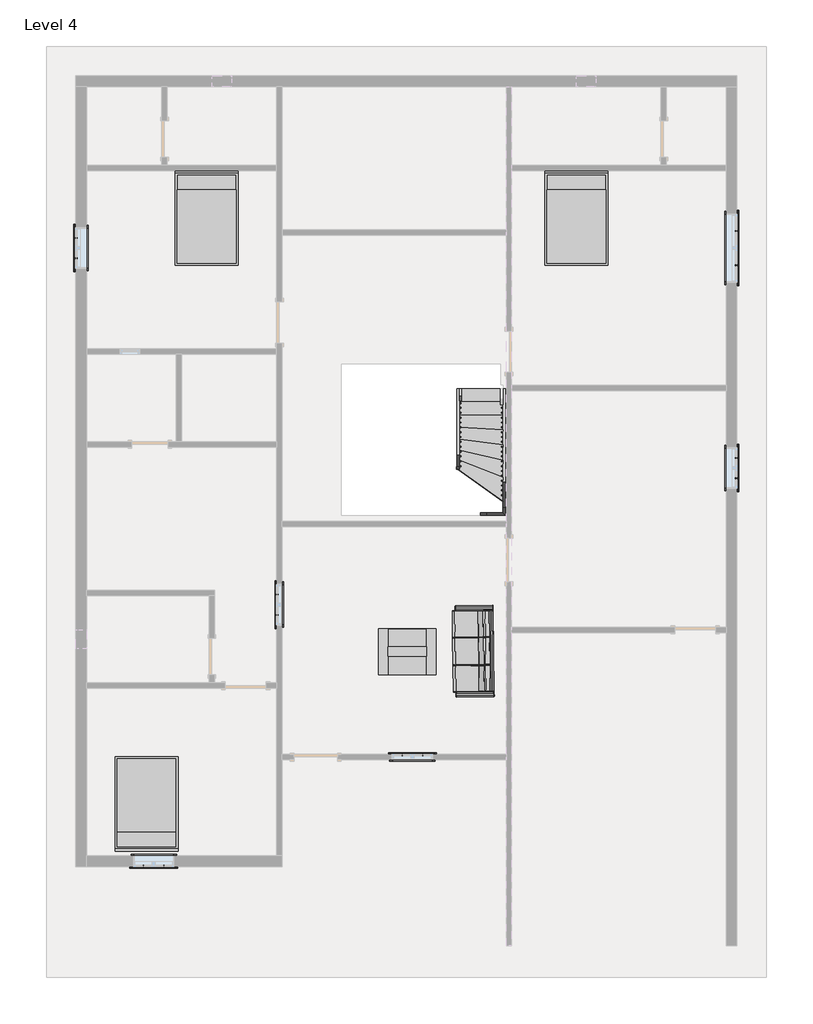
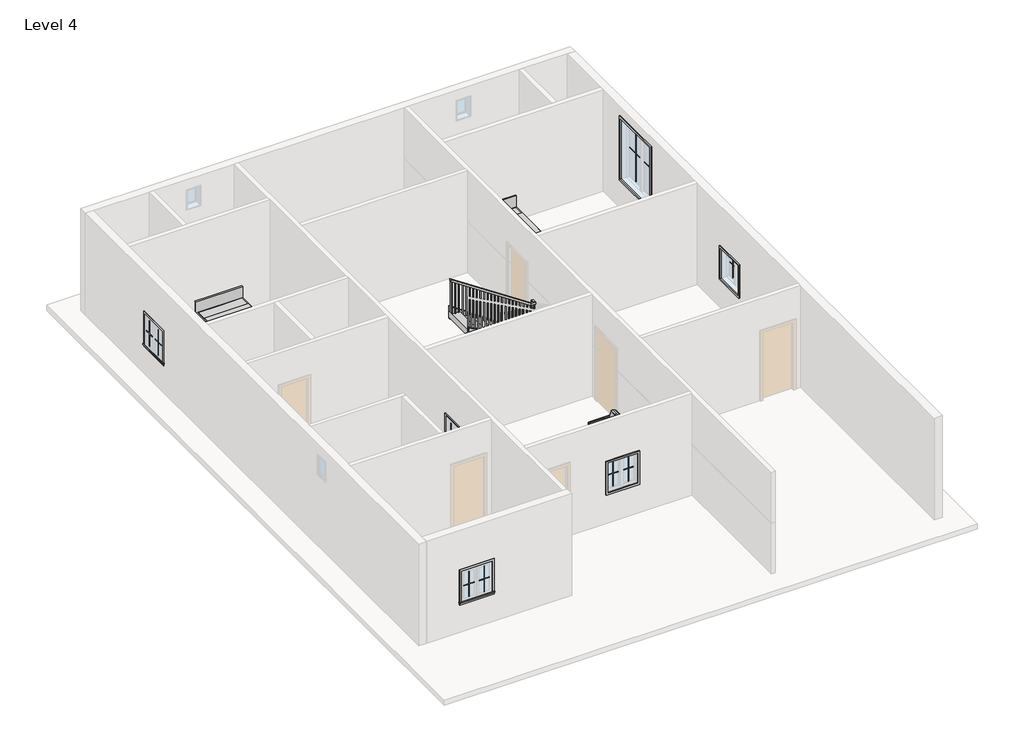
# One storey, part 3 of 3: 24 proxies, 6 members, 5 furniture elements, 1 railing, 1 stair flight.
"""IFC4 building model written with IfcOpenShell, lengths in millimetres."""

from ifc_helpers import new_model, si_unit, frame, origin, place, context, project, spatial, polyline, outline, extrude, faceted_brep, transform, mapped, element, save
from components import muntin_pattern_2x2_muntin_pattern_2x2_b3fe6957, muntin_pattern_2x2_muntin_pattern_2x2_3e0ecaf2, muntin_pattern_2x2_muntin_pattern_2x2_bff912c5, muntin_pattern_2x2_muntin_pattern_2x2_c2194282, trim_window_exterior_flat_with_sill_41619996, trim_window_exterior_flat_with_sill_e04b3088, trim_window_interior_flat_picture_frame_51c85655, trim_window_interior_flat_picture_frame_2a7685fe, furniture_2fc85b74, furniture_29a9adb8, furniture_57072a26, bed_17739_bed_17739_15c61121, wood_and_glass_coffee_table_17065_wood_and_glass_coffee_dbc724b2, stair_flight_9178a8c5

model = new_model("IFC4")

# Units and contexts
model_context = context("Model", 3, world=origin())
ifc_project = project(units=[si_unit("LENGTHUNIT", "METRE", prefix="MILLI")], contexts=[model_context])

# Site, building, storey
site = spatial("IfcSite", under=ifc_project)
building = spatial("IfcBuilding", under=site)
storey = spatial("IfcBuildingStorey", under=building, Name="Level 4", Elevation=6400.8)

# Proxies
placement = place(None, origin())
muntin_pattern_2x2_muntin_pattern_2x2_shape = muntin_pattern_2x2_muntin_pattern_2x2_b3fe6957(model_context)
element("IfcBuildingElementProxy", 1, Name="Muntin Pattern_2x2 : Muntin Pattern_2x2", ObjectType="Muntin Pattern_2x2 : Muntin Pattern_2x2", at=placement, inside=storey, context=model_context, shape_type="MappedRepresentation", body=[
    mapped(muntin_pattern_2x2_muntin_pattern_2x2_shape, transform((-7494.1165084, 6600.4397623, 7385.05), x_axis=(0.0, 1.0, 0.0), y_axis=(-1.0, 0.0, 0.0), z_axis=(0.0, 0.0, 1.0))),
])
element("IfcBuildingElementProxy", 2, Name="Muntin Pattern_2x2 : Muntin Pattern_2x2", ObjectType="Muntin Pattern_2x2 : Muntin Pattern_2x2", at=placement, inside=storey, context=model_context, shape_type="MappedRepresentation", body=[
    mapped(muntin_pattern_2x2_muntin_pattern_2x2_shape, transform((-5651.0290084, -6136.0727377, 7385.05), x_axis=(-1.0, 0.0, 0.0), y_axis=(0.0, -1.0, 0.0), z_axis=(0.0, 0.0, 1.0))),
])
element("IfcBuildingElementProxy", 3, Name="Muntin Pattern_2x2 : Muntin Pattern_2x2", ObjectType="Muntin Pattern_2x2 : Muntin Pattern_2x2", at=placement, inside=storey, context=model_context, shape_type="MappedRepresentation", body=[
    mapped(muntin_pattern_2x2_muntin_pattern_2x2_shape, transform((-656.7540084, -3805.6227377, 7385.05), x_axis=(1.0, 0.0, 0.0), y_axis=(0.0, 1.0, 0.0), z_axis=(0.0, 0.0, 1.0))),
])
element("IfcBuildingElementProxy", 4, Name="Muntin Pattern_2x2 : Muntin Pattern_2x2", ObjectType="Muntin Pattern_2x2 : Muntin Pattern_2x2", at=placement, inside=storey, context=model_context, shape_type="MappedRepresentation", body=[
    mapped(muntin_pattern_2x2_muntin_pattern_2x2_shape, transform((6355.2334916, 2418.9647623, 7385.05), x_axis=(0.0, -1.0, 0.0), y_axis=(1.0, 0.0, 0.0), z_axis=(0.0, 0.0, 1.0))),
])
element("IfcBuildingElementProxy", 5, Name="Muntin Pattern_2x2 : Muntin Pattern_2x2", ObjectType="Muntin Pattern_2x2 : Muntin Pattern_2x2", at=placement, inside=storey, context=model_context, shape_type="MappedRepresentation", body=[
    mapped(muntin_pattern_2x2_muntin_pattern_2x2_shape, transform((-3277.7165084, -873.5102377, 7385.05), x_axis=(0.0, 1.0, 0.0), y_axis=(-1.0, 0.0, 0.0), z_axis=(0.0, 0.0, 1.0))),
])
muntin_pattern_2x2_muntin_pattern_2x2_2_shape = muntin_pattern_2x2_muntin_pattern_2x2_3e0ecaf2(model_context)
element("IfcBuildingElementProxy", 6, Name="Muntin Pattern_2x2 : Muntin Pattern_2x2", ObjectType="Muntin Pattern_2x2 : Muntin Pattern_2x2", at=placement, inside=storey, context=model_context, shape_type="MappedRepresentation", body=[
    mapped(muntin_pattern_2x2_muntin_pattern_2x2_2_shape, transform((-7494.1165084, 7029.0647623, 7385.05), x_axis=(0.0, -1.0, 0.0), y_axis=(1.0, 0.0, 0.0), z_axis=(0.0, 0.0, 1.0))),
])
element("IfcBuildingElementProxy", 7, Name="Muntin Pattern_2x2 : Muntin Pattern_2x2", ObjectType="Muntin Pattern_2x2 : Muntin Pattern_2x2", at=placement, inside=storey, context=model_context, shape_type="MappedRepresentation", body=[
    mapped(muntin_pattern_2x2_muntin_pattern_2x2_2_shape, transform((-6079.6540084, -6136.0727377, 7385.05), x_axis=(1.0, 0.0, 0.0), y_axis=(0.0, 1.0, 0.0), z_axis=(0.0, 0.0, 1.0))),
])
element("IfcBuildingElementProxy", 8, Name="Muntin Pattern_2x2 : Muntin Pattern_2x2", ObjectType="Muntin Pattern_2x2 : Muntin Pattern_2x2", at=placement, inside=storey, context=model_context, shape_type="MappedRepresentation", body=[
    mapped(muntin_pattern_2x2_muntin_pattern_2x2_2_shape, transform((-228.1290084, -3805.6227377, 7385.05), x_axis=(-1.0, 0.0, 0.0), y_axis=(0.0, -1.0, 0.0), z_axis=(0.0, 0.0, 1.0))),
])
element("IfcBuildingElementProxy", 9, Name="Muntin Pattern_2x2 : Muntin Pattern_2x2", ObjectType="Muntin Pattern_2x2 : Muntin Pattern_2x2", at=placement, inside=storey, context=model_context, shape_type="MappedRepresentation", body=[
    mapped(muntin_pattern_2x2_muntin_pattern_2x2_2_shape, transform((6355.2334916, 1990.3397623, 7385.05), x_axis=(0.0, 1.0, 0.0), y_axis=(-1.0, 0.0, 0.0), z_axis=(0.0, 0.0, 1.0))),
])
element("IfcBuildingElementProxy", 10, Name="Muntin Pattern_2x2 : Muntin Pattern_2x2", ObjectType="Muntin Pattern_2x2 : Muntin Pattern_2x2", at=placement, inside=storey, context=model_context, shape_type="MappedRepresentation", body=[
    mapped(muntin_pattern_2x2_muntin_pattern_2x2_2_shape, transform((-3277.7165084, -444.8852377, 7385.05), x_axis=(0.0, -1.0, 0.0), y_axis=(1.0, 0.0, 0.0), z_axis=(0.0, 0.0, 1.0))),
])
muntin_pattern_2x2_muntin_pattern_2x2_3_shape = muntin_pattern_2x2_muntin_pattern_2x2_bff912c5(model_context)
element("IfcBuildingElementProxy", 11, Name="Muntin Pattern_2x2 : Muntin Pattern_2x2", ObjectType="Muntin Pattern_2x2 : Muntin Pattern_2x2", at=placement, inside=storey, context=model_context, shape_type="MappedRepresentation", body=[
    mapped(muntin_pattern_2x2_muntin_pattern_2x2_3_shape, transform((6355.2334916, 7175.1147623, 7385.05), x_axis=(0.0, -1.0, 0.0), y_axis=(1.0, 0.0, 0.0), z_axis=(0.0, 0.0, 1.0))),
])
muntin_pattern_2x2_muntin_pattern_2x2_4_shape = muntin_pattern_2x2_muntin_pattern_2x2_c2194282(model_context)
element("IfcBuildingElementProxy", 12, Name="Muntin Pattern_2x2 : Muntin Pattern_2x2", ObjectType="Muntin Pattern_2x2 : Muntin Pattern_2x2", at=placement, inside=storey, context=model_context, shape_type="MappedRepresentation", body=[
    mapped(muntin_pattern_2x2_muntin_pattern_2x2_4_shape, transform((6355.2334916, 6454.3897623, 7385.05), x_axis=(0.0, 1.0, 0.0), y_axis=(-1.0, 0.0, 0.0), z_axis=(0.0, 0.0, 1.0))),
])
trim_window_exterior_flat_with_sill_shape = trim_window_exterior_flat_with_sill_41619996(model_context)
element("IfcBuildingElementProxy", 13, Name="Trim-Window-Exterior-Flat : with Sill", ObjectType="Trim-Window-Exterior-Flat : with Sill", at=placement, inside=storey, context=model_context, shape_type="MappedRepresentation", body=[
    mapped(trim_window_exterior_flat_with_sill_shape, transform((-7503.6415084, 6814.7522623, 8229.6), x_axis=(0.0, -1.0, 0.0), y_axis=(0.0, 0.0, 1.0), z_axis=(-1.0, 0.0, 0.0))),
])
element("IfcBuildingElementProxy", 14, Name="Trim-Window-Exterior-Flat : with Sill", ObjectType="Trim-Window-Exterior-Flat : with Sill", at=placement, inside=storey, context=model_context, shape_type="MappedRepresentation", body=[
    mapped(trim_window_exterior_flat_with_sill_shape, transform((-5865.3415084, -6145.5977377, 8229.6), x_axis=(1.0, 0.0, 0.0), y_axis=(0.0, 0.0, 1.0), z_axis=(0.0, -1.0, 0.0))),
])
element("IfcBuildingElementProxy", 15, Name="Trim-Window-Exterior-Flat : with Sill", ObjectType="Trim-Window-Exterior-Flat : with Sill", at=placement, inside=storey, context=model_context, shape_type="MappedRepresentation", body=[
    mapped(trim_window_exterior_flat_with_sill_shape, transform((-442.4415084, -3796.0977377, 8229.6), x_axis=(-1.0, 0.0, 0.0), y_axis=(0.0, 0.0, 1.0), z_axis=(0.0, 1.0, 0.0))),
])
element("IfcBuildingElementProxy", 16, Name="Trim-Window-Exterior-Flat : with Sill", ObjectType="Trim-Window-Exterior-Flat : with Sill", at=placement, inside=storey, context=model_context, shape_type="MappedRepresentation", body=[
    mapped(trim_window_exterior_flat_with_sill_shape, transform((6364.7584916, 2204.6522623, 8229.6), x_axis=(0.0, 1.0, 0.0), y_axis=(0.0, 0.0, 1.0), z_axis=(1.0, 0.0, 0.0))),
])
element("IfcBuildingElementProxy", 17, Name="Trim-Window-Exterior-Flat : with Sill", ObjectType="Trim-Window-Exterior-Flat : with Sill", at=placement, inside=storey, context=model_context, shape_type="MappedRepresentation", body=[
    mapped(trim_window_exterior_flat_with_sill_shape, transform((-3287.2415084, -659.1977377, 8229.6), x_axis=(0.0, -1.0, 0.0), y_axis=(0.0, 0.0, 1.0), z_axis=(-1.0, 0.0, 0.0))),
])
trim_window_exterior_flat_with_sill_2_shape = trim_window_exterior_flat_with_sill_e04b3088(model_context)
element("IfcBuildingElementProxy", 18, Name="Trim-Window-Exterior-Flat : with Sill", ObjectType="Trim-Window-Exterior-Flat : with Sill", at=placement, inside=storey, context=model_context, shape_type="MappedRepresentation", body=[
    mapped(trim_window_exterior_flat_with_sill_2_shape, transform((6364.7584916, 6814.7522623, 9144.0), x_axis=(0.0, 1.0, 0.0), y_axis=(0.0, 0.0, 1.0), z_axis=(1.0, 0.0, 0.0))),
])
trim_window_interior_flat_picture_frame_shape = trim_window_interior_flat_picture_frame_51c85655(model_context)
element("IfcBuildingElementProxy", 19, Name="Trim-Window-Interior-Flat : Picture Frame", ObjectType="Trim-Window-Interior-Flat : Picture Frame", at=placement, inside=storey, context=model_context, shape_type="MappedRepresentation", body=[
    mapped(trim_window_interior_flat_picture_frame_shape, transform((-7275.0415084, 6814.7522623, 8229.6), x_axis=(0.0, 1.0, 0.0), y_axis=(0.0, 0.0, 1.0), z_axis=(1.0, 0.0, 0.0))),
])
element("IfcBuildingElementProxy", 20, Name="Trim-Window-Interior-Flat : Picture Frame", ObjectType="Trim-Window-Interior-Flat : Picture Frame", at=placement, inside=storey, context=model_context, shape_type="MappedRepresentation", body=[
    mapped(trim_window_interior_flat_picture_frame_shape, transform((-5865.3415084, -5916.9977377, 8229.6), x_axis=(-1.0, 0.0, 0.0), y_axis=(0.0, 0.0, 1.0), z_axis=(0.0, 1.0, 0.0))),
])
element("IfcBuildingElementProxy", 21, Name="Trim-Window-Interior-Flat : Picture Frame", ObjectType="Trim-Window-Interior-Flat : Picture Frame", at=placement, inside=storey, context=model_context, shape_type="MappedRepresentation", body=[
    mapped(trim_window_interior_flat_picture_frame_shape, transform((-442.4415084, -3910.3977377, 8229.6), x_axis=(1.0, 0.0, 0.0), y_axis=(0.0, 0.0, 1.0), z_axis=(0.0, -1.0, 0.0))),
])
element("IfcBuildingElementProxy", 22, Name="Trim-Window-Interior-Flat : Picture Frame", ObjectType="Trim-Window-Interior-Flat : Picture Frame", at=placement, inside=storey, context=model_context, shape_type="MappedRepresentation", body=[
    mapped(trim_window_interior_flat_picture_frame_shape, transform((6136.1584916, 2204.6522623, 8229.6), x_axis=(0.0, -1.0, 0.0), y_axis=(0.0, 0.0, 1.0), z_axis=(-1.0, 0.0, 0.0))),
])
element("IfcBuildingElementProxy", 23, Name="Trim-Window-Interior-Flat : Picture Frame", ObjectType="Trim-Window-Interior-Flat : Picture Frame", at=placement, inside=storey, context=model_context, shape_type="MappedRepresentation", body=[
    mapped(trim_window_interior_flat_picture_frame_shape, transform((-3172.9415084, -659.1977377, 8229.6), x_axis=(0.0, 1.0, 0.0), y_axis=(0.0, 0.0, 1.0), z_axis=(1.0, 0.0, 0.0))),
])
trim_window_interior_flat_picture_frame_2_shape = trim_window_interior_flat_picture_frame_2a7685fe(model_context)
element("IfcBuildingElementProxy", 24, Name="Trim-Window-Interior-Flat : Picture Frame", ObjectType="Trim-Window-Interior-Flat : Picture Frame", at=placement, inside=storey, context=model_context, shape_type="MappedRepresentation", body=[
    mapped(trim_window_interior_flat_picture_frame_2_shape, transform((6136.1584916, 6814.7522623, 9144.0), x_axis=(0.0, -1.0, 0.0), y_axis=(0.0, 0.0, 1.0), z_axis=(-1.0, 0.0, 0.0))),
])

# Furniture
furniture_shape = furniture_2fc85b74(model_context)
furniture_2_shape = furniture_29a9adb8(model_context)
furniture_3_shape = furniture_57072a26(model_context)
element("IfcFurniture", 25, at=placement, inside=storey, context=model_context, shape_type="MappedRepresentation", body=[
    mapped(furniture_shape, transform((460.7695276, -1640.1238257, 6400.8), x_axis=(0.014042050983927294, -0.9999014055416489, 0.0), y_axis=(0.9999014055416489, 0.014042050983927294, 0.0), z_axis=(0.0, 0.0, 1.0))),
    mapped(furniture_2_shape, transform((460.7695276, -1640.1238257, 6400.8), x_axis=(0.014042050983927294, -0.9999014055416489, 0.0), y_axis=(0.9999014055416489, 0.014042050983927294, 0.0), z_axis=(0.0, 0.0, 1.0))),
    mapped(furniture_3_shape, transform((460.7695276, -1640.1238257, 6400.8), x_axis=(0.014042050983927294, -0.9999014055416489, 0.0), y_axis=(0.9999014055416489, 0.014042050983927294, 0.0), z_axis=(0.0, 0.0, 1.0))),
])
bed_17739_bed_17739_shape = bed_17739_bed_17739_15c61121(model_context)
element("IfcFurniture", 26, ObjectType="Bed_17739 : Bed_17739", at=placement, inside=storey, context=model_context, shape_type="MappedRepresentation", body=[
    mapped(bed_17739_bed_17739_shape, transform((-4754.0915084, 7424.3522623, 6400.8), x_axis=(1.0, 0.0, 0.0), y_axis=(0.0, 1.0, 0.0), z_axis=(0.0, 0.0, 1.0))),
])
element("IfcFurniture", 27, ObjectType="Bed_17739 : Bed_17739", at=placement, inside=storey, context=model_context, shape_type="MappedRepresentation", body=[
    mapped(bed_17739_bed_17739_shape, transform((2998.5366507, 7424.3522623, 6400.8), x_axis=(1.0, 0.0, 0.0), y_axis=(0.0, 1.0, 0.0), z_axis=(0.0, 0.0, 1.0))),
])
element("IfcFurniture", 28, ObjectType="Bed_17739 : Bed_17739", at=placement, inside=storey, context=model_context, shape_type="MappedRepresentation", body=[
    mapped(bed_17739_bed_17739_shape, transform((-6017.7415084, -4812.0977377, 6400.8), x_axis=(-1.0, 0.0, 0.0), y_axis=(0.0, -1.0, 0.0), z_axis=(0.0, 0.0, 1.0))),
])
wood_and_glass_coffee_table_17065_wood_and_glass_coffee_shape = wood_and_glass_coffee_table_17065_wood_and_glass_coffee_dbc724b2(model_context)
element("IfcFurniture", 29, ObjectType="Wood_and_Glass_Coffee_Table_17065 : Wood_and_Glass_Coffee_Table_17065", at=placement, inside=storey, context=model_context, shape_type="MappedRepresentation", body=[
    mapped(wood_and_glass_coffee_table_17065_wood_and_glass_coffee_shape, transform((-550.3915084, -1643.4477377, 6400.8), x_axis=(1.0, 0.0, 0.0), y_axis=(0.0, 1.0, 0.0), z_axis=(0.0, 0.0, 1.0))),
])

# Members
element("IfcMember", 30, ObjectType="Stringer - 2\" Width", at=placement, inside=storey, context=model_context, shape_type="SweptSolid", body=[
    extrude(outline(polyline([(3870.4222402, 6634.4789033), (3870.4222402, 6400.8), (3655.4968958, 6400.8), (1369.1992084, 7533.4067011), (1369.1992084, 7873.5572536), (3870.4222402, 6634.4789033)])), frame((1456.2084916, 0.0, 0.0), z_axis=(1.0, 0.0, 0.0), x_axis=(0.0, 1.0, 0.0)), (0.0, 0.0, 1.0), 50.8),
])
element("IfcMember", 31, ObjectType="Stringer - 2\" Width", at=placement, inside=storey, context=model_context, shape_type="SweptSolid", body=[
    extrude(outline(polyline([(1456.2084916, 1369.1992084), (1507.0084916, 1369.1992084), (1507.0084916, 1218.1652728), (1456.2084916, 1268.9652728), (1456.2084916, 1369.1992084)])), frame((0.0, 0.0, 7533.4067011), z_axis=(0.0, 0.0, 1.0), x_axis=(1.0, 0.0, 0.0)), (0.0, 0.0, 1.0), 340.1505525),
])
element("IfcMember", 32, ObjectType="Stringer - 2\" Width", at=placement, inside=storey, context=model_context, shape_type="SweptSolid", body=[
    extrude(outline(polyline([(1456.2084916, 1268.9652728), (1507.0084916, 1218.1652728), (1113.208453, 1218.1652728), (1113.208453, 1268.9652728), (1456.2084916, 1268.9652728)])), frame((0.0, 0.0, 7533.4067011), z_axis=(0.0, 0.0, 1.0), x_axis=(1.0, 0.0, 0.0)), (0.0, 0.0, 1.0), 340.1505525),
])
element("IfcMember", 33, ObjectType="Stringer - 2\" Width", at=placement, inside=storey, context=model_context, shape_type="SweptSolid", body=[
    extrude(outline(polyline([(3870.4222402, 6591.0545013), (3870.4222402, 6400.8), (3614.0281198, 6400.8), (2234.1652728, 7407.2313584), (2234.1652728, 7784.4921868), (3870.4222402, 6591.0545013)])), frame((491.0084916, 0.0, 0.0), z_axis=(1.0, 0.0, 0.0), x_axis=(0.0, 1.0, 0.0)), (0.0, 0.0, 1.0), 50.8),
])
element("IfcMember", 34, ObjectType="Stringer - 2\" Width", at=placement, inside=storey, context=model_context, shape_type="SweptSolid", body=[
    extrude(outline(polyline([(7558.9835681, 541.8084916), (7926.7965617, 541.8084916), (9517.7897736, -1813.7050583), (9149.97678, -1813.7050583), (7558.9835681, 541.8084916)])), frame((0.0, 2183.3652728, 0.0), z_axis=(0.0, 1.0, 0.0), x_axis=(0.0, 0.0, 1.0)), (0.0, 0.0, 1.0), 50.8),
])
element("IfcMember", 35, ObjectType="Stringer - 2\" Width", at=placement, inside=storey, context=model_context, shape_type="SweptSolid", body=[
    extrude(outline(polyline([(7533.4067011, 1113.208453), (7873.5572536, 1113.208453), (9464.7877281, -1813.7050583), (9124.6371756, -1813.7050583), (7533.4067011, 1113.208453)])), frame((0.0, 1218.1652728, 0.0), z_axis=(0.0, 1.0, 0.0), x_axis=(0.0, 0.0, 1.0)), (0.0, 0.0, 1.0), 50.8),
])

# Railing
element("IfcRailing", 36, ObjectType="Handrail - Rectangular", at=placement, inside=storey, context=model_context, shape_type="SolidModel", body=[
    faceted_brep([(592.6084916, 3870.4222402, 7484.5333333), (592.6084916, 3870.4222402, 7422.2674881), (541.8084916, 3870.4222402, 7422.2674881), (541.8084916, 3870.4222402, 7484.5333333), (592.6084916, 2259.5652728, 8626.2596781), (592.6084916, 2208.7652728, 8599.9993253), (541.8084916, 2208.7652728, 8599.9993253), (541.8084916, 2259.5652728, 8626.2596781), (592.6084916, 2259.5652728, 8843.0092282), (592.6084916, 2208.7652728, 8792.2092282), (541.8084916, 2208.7652728, 8792.2092282), (541.8084916, 2259.5652728, 8843.0092282), (592.6084916, 2132.5652728, 8843.0092282), (592.6084916, 2132.5652728, 8792.2092282), (541.8084916, 2183.3652728, 8792.2092282), (541.8084916, 2183.3652728, 8843.0092282), (465.6084916, 2132.5652728, 8843.0092282), (450.2220288, 2132.5652728, 8792.2092282), (450.2220288, 2183.3652728, 8792.2092282), (465.6084916, 2183.3652728, 8843.0092282), (-1813.7050583, 2132.5652728, 10363.2), (-1813.7050583, 2183.3652728, 10363.2), (-1813.7050583, 2183.3652728, 10302.1379811), (-1813.7050583, 2132.5652728, 10302.1379811)], [[[0, 1, 2, 3]], [[1, 0, 4, 5]], [[2, 1, 5, 6]], [[3, 2, 6, 7]], [[0, 3, 7, 4]], [[5, 4, 8, 9]], [[6, 5, 9, 10]], [[7, 6, 10, 11]], [[4, 7, 11, 8]], [[9, 8, 12, 13]], [[10, 9, 13, 14]], [[11, 10, 14, 15]], [[8, 11, 15, 12]], [[13, 12, 16, 17]], [[14, 13, 17, 18]], [[15, 14, 18, 19]], [[12, 15, 19, 16]], [[20, 21, 22, 23]], [[17, 16, 20, 23]], [[18, 17, 23, 22]], [[19, 18, 22, 21]], [[16, 19, 21, 20]]]),
    extrude(outline(polyline([(10266.3636891, -1760.0665084), (10279.0691083, -1779.1165084), (9279.4666667, -1779.1165084), (9279.4666667, -1760.0665084), (10266.3636891, -1760.0665084)])), frame((0.0, 2148.4402728, 0.0), z_axis=(0.0, 1.0, 0.0), x_axis=(0.0, 0.0, 1.0)), (0.0, 0.0, 1.0), 19.05),
    extrude(outline(polyline([(10198.6014532, -1658.4665084), (10211.3068724, -1677.5165084), (9279.4666667, -1677.5165084), (9279.4666667, -1658.4665084), (10198.6014532, -1658.4665084)])), frame((0.0, 2148.4402728, 0.0), z_axis=(0.0, 1.0, 0.0), x_axis=(0.0, 0.0, 1.0)), (0.0, 0.0, 1.0), 19.05),
    extrude(outline(polyline([(10130.8392173, -1556.8665084), (10143.5446365, -1575.9165084), (9279.4666667, -1575.9165084), (9279.4666667, -1556.8665084), (10130.8392173, -1556.8665084)])), frame((0.0, 2148.4402728, 0.0), z_axis=(0.0, 1.0, 0.0), x_axis=(0.0, 0.0, 1.0)), (0.0, 0.0, 1.0), 19.05),
    extrude(outline(polyline([(10062.9324687, -1455.2665084), (10075.6378879, -1474.3165084), (9110.1333333, -1474.3165084), (9110.1333333, -1455.2665084), (10062.9324687, -1455.2665084)])), frame((0.0, 2148.4402728, 0.0), z_axis=(0.0, 1.0, 0.0), x_axis=(0.0, 0.0, 1.0)), (0.0, 0.0, 1.0), 19.05),
    extrude(outline(polyline([(9995.1702328, -1353.6665084), (10007.875652, -1372.7165084), (9110.1333333, -1372.7165084), (9110.1333333, -1353.6665084), (9995.1702328, -1353.6665084)])), frame((0.0, 2148.4402728, 0.0), z_axis=(0.0, 1.0, 0.0), x_axis=(0.0, 0.0, 1.0)), (0.0, 0.0, 1.0), 19.05),
    extrude(outline(polyline([(9927.4079969, -1252.0665084), (9940.1134161, -1271.1165084), (9110.1333333, -1271.1165084), (9110.1333333, -1252.0665084), (9927.4079969, -1252.0665084)])), frame((0.0, 2148.4402728, 0.0), z_axis=(0.0, 1.0, 0.0), x_axis=(0.0, 0.0, 1.0)), (0.0, 0.0, 1.0), 19.05),
    extrude(outline(polyline([(9859.645761, -1150.4665084), (9872.3511802, -1169.5165084), (8940.8, -1169.5165084), (8940.8, -1150.4665084), (9859.645761, -1150.4665084)])), frame((0.0, 2148.4402728, 0.0), z_axis=(0.0, 1.0, 0.0), x_axis=(0.0, 0.0, 1.0)), (0.0, 0.0, 1.0), 19.05),
    extrude(outline(polyline([(9791.8835251, -1048.8665084), (9804.5889444, -1067.9165084), (8940.8, -1067.9165084), (8940.8, -1048.8665084), (9791.8835251, -1048.8665084)])), frame((0.0, 2148.4402728, 0.0), z_axis=(0.0, 1.0, 0.0), x_axis=(0.0, 0.0, 1.0)), (0.0, 0.0, 1.0), 19.05),
    extrude(outline(polyline([(9724.265802, -947.2665084), (9736.9712212, -966.3165084), (8771.4666667, -966.3165084), (8771.4666667, -947.2665084), (9724.265802, -947.2665084)])), frame((0.0, 2148.4402728, 0.0), z_axis=(0.0, 1.0, 0.0), x_axis=(0.0, 0.0, 1.0)), (0.0, 0.0, 1.0), 19.05),
    extrude(outline(polyline([(9656.5035661, -845.6665084), (9669.2089853, -864.7165084), (8771.4666667, -864.7165084), (8771.4666667, -845.6665084), (9656.5035661, -845.6665084)])), frame((0.0, 2148.4402728, 0.0), z_axis=(0.0, 1.0, 0.0), x_axis=(0.0, 0.0, 1.0)), (0.0, 0.0, 1.0), 19.05),
    extrude(outline(polyline([(9588.7413302, -744.0665084), (9601.4467495, -763.1165084), (8771.4666667, -763.1165084), (8771.4666667, -744.0665084), (9588.7413302, -744.0665084)])), frame((0.0, 2148.4402728, 0.0), z_axis=(0.0, 1.0, 0.0), x_axis=(0.0, 0.0, 1.0)), (0.0, 0.0, 1.0), 19.05),
    extrude(outline(polyline([(9520.9790943, -642.4665084), (9533.6845136, -661.5165084), (8602.1333333, -661.5165084), (8602.1333333, -642.4665084), (9520.9790943, -642.4665084)])), frame((0.0, 2148.4402728, 0.0), z_axis=(0.0, 1.0, 0.0), x_axis=(0.0, 0.0, 1.0)), (0.0, 0.0, 1.0), 19.05),
    extrude(outline(polyline([(9453.2168585, -540.8665084), (9465.9222777, -559.9165084), (8602.1333333, -559.9165084), (8602.1333333, -540.8665084), (9453.2168585, -540.8665084)])), frame((0.0, 2148.4402728, 0.0), z_axis=(0.0, 1.0, 0.0), x_axis=(0.0, 0.0, 1.0)), (0.0, 0.0, 1.0), 19.05),
    extrude(outline(polyline([(9385.3101098, -439.2665084), (9398.0155291, -458.3165084), (8602.1333333, -458.3165084), (8602.1333333, -439.2665084), (9385.3101098, -439.2665084)])), frame((0.0, 2148.4402728, 0.0), z_axis=(0.0, 1.0, 0.0), x_axis=(0.0, 0.0, 1.0)), (0.0, 0.0, 1.0), 19.05),
    extrude(outline(polyline([(9317.5478739, -337.6665084), (9330.2532932, -356.7165084), (8432.8, -356.7165084), (8432.8, -337.6665084), (9317.5478739, -337.6665084)])), frame((0.0, 2148.4402728, 0.0), z_axis=(0.0, 1.0, 0.0), x_axis=(0.0, 0.0, 1.0)), (0.0, 0.0, 1.0), 19.05),
    extrude(outline(polyline([(9249.7856381, -236.0665084), (9262.4910573, -255.1165084), (8432.8, -255.1165084), (8432.8, -236.0665084), (9249.7856381, -236.0665084)])), frame((0.0, 2148.4402728, 0.0), z_axis=(0.0, 1.0, 0.0), x_axis=(0.0, 0.0, 1.0)), (0.0, 0.0, 1.0), 19.05),
    extrude(outline(polyline([(9182.0234022, -134.4665084), (9194.7288214, -153.5165084), (8263.4666667, -153.5165084), (8263.4666667, -134.4665084), (9182.0234022, -134.4665084)])), frame((0.0, 2148.4402728, 0.0), z_axis=(0.0, 1.0, 0.0), x_axis=(0.0, 0.0, 1.0)), (0.0, 0.0, 1.0), 19.05),
    extrude(outline(polyline([(9114.2611663, -32.8665084), (9126.9665855, -51.9165084), (8263.4666667, -51.9165084), (8263.4666667, -32.8665084), (9114.2611663, -32.8665084)])), frame((0.0, 2148.4402728, 0.0), z_axis=(0.0, 1.0, 0.0), x_axis=(0.0, 0.0, 1.0)), (0.0, 0.0, 1.0), 19.05),
    extrude(outline(polyline([(9046.6434432, 68.7334916), (9059.3488624, 49.6834916), (8263.4666667, 49.6834916), (8263.4666667, 68.7334916), (9046.6434432, 68.7334916)])), frame((0.0, 2148.4402728, 0.0), z_axis=(0.0, 1.0, 0.0), x_axis=(0.0, 0.0, 1.0)), (0.0, 0.0, 1.0), 19.05),
    extrude(outline(polyline([(8978.8812073, 170.3334916), (8991.5866265, 151.2834916), (8094.1333333, 151.2834916), (8094.1333333, 170.3334916), (8978.8812073, 170.3334916)])), frame((0.0, 2148.4402728, 0.0), z_axis=(0.0, 1.0, 0.0), x_axis=(0.0, 0.0, 1.0)), (0.0, 0.0, 1.0), 19.05),
    extrude(outline(polyline([(8911.1189714, 271.9334916), (8923.8243906, 252.8834916), (8094.1333333, 252.8834916), (8094.1333333, 271.9334916), (8911.1189714, 271.9334916)])), frame((0.0, 2148.4402728, 0.0), z_axis=(0.0, 1.0, 0.0), x_axis=(0.0, 0.0, 1.0)), (0.0, 0.0, 1.0), 19.05),
    extrude(outline(polyline([(8843.3567355, 373.5334916), (8856.0621547, 354.4834916), (7924.8, 354.4834916), (7924.8, 373.5334916), (8843.3567355, 373.5334916)])), frame((0.0, 2148.4402728, 0.0), z_axis=(0.0, 1.0, 0.0), x_axis=(0.0, 0.0, 1.0)), (0.0, 0.0, 1.0), 19.05),
    extrude(outline(polyline([(8775.5944996, 475.1334916), (8788.2999189, 456.0834916), (7924.8, 456.0834916), (7924.8, 475.1334916), (8775.5944996, 475.1334916)])), frame((0.0, 2148.4402728, 0.0), z_axis=(0.0, 1.0, 0.0), x_axis=(0.0, 0.0, 1.0)), (0.0, 0.0, 1.0), 19.05),
    extrude(outline(polyline([(557.6834916, 2254.3472402), (576.7334916, 2254.3472402), (576.7334916, 2235.2972402), (557.6834916, 2235.2972402), (557.6834916, 2254.3472402)])), frame((0.0, 0.0, 7586.1333333), z_axis=(0.0, 0.0, 1.0), x_axis=(1.0, 0.0, 0.0)), (0.0, 0.0, 1.0), 1206.0758948),
    extrude(outline(polyline([(2336.8972402, 8509.1832902), (2355.9472402, 8495.6812306), (2355.9472402, 7586.1333333), (2336.8972402, 7586.1333333), (2336.8972402, 8509.1832902)])), frame((557.6834916, 0.0, 0.0), z_axis=(1.0, 0.0, 0.0), x_axis=(0.0, 1.0, 0.0)), (0.0, 0.0, 1.0), 19.05),
    extrude(outline(polyline([(2438.4972402, 8437.1723054), (2457.5472402, 8423.6702458), (2457.5472402, 7416.8), (2438.4972402, 7416.8), (2438.4972402, 8437.1723054)])), frame((557.6834916, 0.0, 0.0), z_axis=(1.0, 0.0, 0.0), x_axis=(0.0, 1.0, 0.0)), (0.0, 0.0, 1.0), 19.05),
    extrude(outline(polyline([(2540.0972402, 8365.1613206), (2559.1472402, 8351.6592609), (2559.1472402, 7416.8), (2540.0972402, 7416.8), (2540.0972402, 8365.1613206)])), frame((557.6834916, 0.0, 0.0), z_axis=(1.0, 0.0, 0.0), x_axis=(0.0, 1.0, 0.0)), (0.0, 0.0, 1.0), 19.05),
    extrude(outline(polyline([(2641.6972402, 8293.1503358), (2660.7472402, 8279.6482761), (2660.7472402, 7247.4666667), (2641.6972402, 7247.4666667), (2641.6972402, 8293.1503358)])), frame((557.6834916, 0.0, 0.0), z_axis=(1.0, 0.0, 0.0), x_axis=(0.0, 1.0, 0.0)), (0.0, 0.0, 1.0), 19.05),
    extrude(outline(polyline([(2743.2972402, 8221.139351), (2762.3472402, 8207.6372913), (2762.3472402, 7247.4666667), (2743.2972402, 7247.4666667), (2743.2972402, 8221.139351)])), frame((557.6834916, 0.0, 0.0), z_axis=(1.0, 0.0, 0.0), x_axis=(0.0, 1.0, 0.0)), (0.0, 0.0, 1.0), 19.05),
    extrude(outline(polyline([(2844.8972402, 8149.1283661), (2863.9472402, 8135.6263065), (2863.9472402, 7078.1333333), (2844.8972402, 7078.1333333), (2844.8972402, 8149.1283661)])), frame((557.6834916, 0.0, 0.0), z_axis=(1.0, 0.0, 0.0), x_axis=(0.0, 1.0, 0.0)), (0.0, 0.0, 1.0), 19.05),
    extrude(outline(polyline([(2946.4972402, 8077.1173813), (2965.5472402, 8063.6153217), (2965.5472402, 7078.1333333), (2946.4972402, 7078.1333333), (2946.4972402, 8077.1173813)])), frame((557.6834916, 0.0, 0.0), z_axis=(1.0, 0.0, 0.0), x_axis=(0.0, 1.0, 0.0)), (0.0, 0.0, 1.0), 19.05),
    extrude(outline(polyline([(3048.0972402, 8005.1063965), (3067.1472402, 7991.6043368), (3067.1472402, 6908.8), (3048.0972402, 6908.8), (3048.0972402, 8005.1063965)])), frame((557.6834916, 0.0, 0.0), z_axis=(1.0, 0.0, 0.0), x_axis=(0.0, 1.0, 0.0)), (0.0, 0.0, 1.0), 19.05),
    extrude(outline(polyline([(3149.6972402, 7933.0954117), (3168.7472402, 7919.593352), (3168.7472402, 6908.8), (3149.6972402, 6908.8), (3149.6972402, 7933.0954117)])), frame((557.6834916, 0.0, 0.0), z_axis=(1.0, 0.0, 0.0), x_axis=(0.0, 1.0, 0.0)), (0.0, 0.0, 1.0), 19.05),
    extrude(outline(polyline([(3251.2972402, 7861.0844268), (3270.3472402, 7847.5823672), (3270.3472402, 6908.8), (3251.2972402, 6908.8), (3251.2972402, 7861.0844268)])), frame((557.6834916, 0.0, 0.0), z_axis=(1.0, 0.0, 0.0), x_axis=(0.0, 1.0, 0.0)), (0.0, 0.0, 1.0), 19.05),
    extrude(outline(polyline([(3352.8972402, 7789.073442), (3371.9472402, 7775.5713824), (3371.9472402, 6739.4666667), (3352.8972402, 6739.4666667), (3352.8972402, 7789.073442)])), frame((557.6834916, 0.0, 0.0), z_axis=(1.0, 0.0, 0.0), x_axis=(0.0, 1.0, 0.0)), (0.0, 0.0, 1.0), 19.05),
    extrude(outline(polyline([(3454.4972402, 7717.0624572), (3473.5472402, 7703.5603975), (3473.5472402, 6739.4666667), (3454.4972402, 6739.4666667), (3454.4972402, 7717.0624572)])), frame((557.6834916, 0.0, 0.0), z_axis=(1.0, 0.0, 0.0), x_axis=(0.0, 1.0, 0.0)), (0.0, 0.0, 1.0), 19.05),
    extrude(outline(polyline([(3556.0972402, 7645.0514724), (3575.1472402, 7631.5494127), (3575.1472402, 6739.4666667), (3556.0972402, 6739.4666667), (3556.0972402, 7645.0514724)])), frame((557.6834916, 0.0, 0.0), z_axis=(1.0, 0.0, 0.0), x_axis=(0.0, 1.0, 0.0)), (0.0, 0.0, 1.0), 19.05),
    extrude(outline(polyline([(3657.6972402, 7573.0404876), (3676.7472402, 7559.5384279), (3676.7472402, 6570.1333333), (3657.6972402, 6570.1333333), (3657.6972402, 7573.0404876)])), frame((557.6834916, 0.0, 0.0), z_axis=(1.0, 0.0, 0.0), x_axis=(0.0, 1.0, 0.0)), (0.0, 0.0, 1.0), 19.05),
    extrude(outline(polyline([(3759.2972402, 7501.0295027), (3778.3472402, 7487.5274431), (3778.3472402, 6570.1333333), (3759.2972402, 6570.1333333), (3759.2972402, 7501.0295027)])), frame((557.6834916, 0.0, 0.0), z_axis=(1.0, 0.0, 0.0), x_axis=(0.0, 1.0, 0.0)), (0.0, 0.0, 1.0), 19.05),
    extrude(outline(polyline([(557.6834916, 2167.4902728), (576.7334916, 2167.4902728), (576.7334916, 2148.4402728), (557.6834916, 2148.4402728), (557.6834916, 2167.4902728)])), frame((0.0, 0.0, 7755.4666667), z_axis=(0.0, 0.0, 1.0), x_axis=(1.0, 0.0, 0.0)), (0.0, 0.0, 1.0), 1036.7425615),
    extrude(outline(polyline([(10289.4325619, -1794.6550583), (10302.1379811, -1813.7050583), (9279.4666667, -1813.7050583), (9279.4666667, -1794.6550583), (10289.4325619, -1794.6550583)])), frame((0.0, 2148.4402728, 0.0), z_axis=(0.0, 1.0, 0.0), x_axis=(0.0, 0.0, 1.0)), (0.0, 0.0, 1.0), 19.05),
    extrude(outline(polyline([(3851.3722402, 7435.7695477), (3870.4222402, 7422.2674881), (3870.4222402, 6570.1333333), (3851.3722402, 6570.1333333), (3851.3722402, 7435.7695477)])), frame((557.6834916, 0.0, 0.0), z_axis=(1.0, 0.0, 0.0), x_axis=(0.0, 1.0, 0.0)), (0.0, 0.0, 1.0), 19.05),
])

# Stair flight
stair_flight_shape = stair_flight_9178a8c5(model_context)
element("IfcStairFlight", 37, ObjectType="2\" Tread 1\" Nosing 1/4\" Riser", at=placement, inside=storey, context=model_context, shape_type="MappedRepresentation", body=[
    mapped(stair_flight_shape, transform((0.0, 0.0, 0.0), x_axis=(1.0, 0.0, 0.0), y_axis=(0.0, 1.0, 0.0), z_axis=(0.0, 0.0, 1.0))),
])

save(model, "model.ifc")

# Revit data of these elements
# Type "Muntin Pattern_2x2 : Muntin Pattern_2x2"
#   Width [instance default] = 4' - 0"
#   Thickness = 0' - 0 1/2"
#   Height [instance default] = 4' - 0"
#   Distance = 0' - 0 3/4"
#   Interior Material [instance default] = none
#   Exterior Material [instance default] = none
#   Default Elevation = 0
# Type "Trim-Window-Exterior-Flat : with Sill"
#   Trim Width = 0' - 2 1/4"
#   Trim Thickness_Picture Frame = 0' - 1 1/4"
#   Trim Thickness_with Sill = 0' - 0 3/4"
#   Sill Thickness = 0' - 1 1/4"
#   Opening Width [instance default] = 2' - 0"
#   Opening Height [instance default] = 3' - 0"
#   Default Elevation = 4' - 0"
#   Sill = yes
#   Picture Frame = no
#   Trim Material [instance default] = none
# Type "Trim-Window-Interior-Flat : Picture Frame"
#   Trim Thickness_Picture Frame = 0' - 1 1/4"
#   Trim Width = 0' - 2 1/4"
#   Trim Thickness_with Sill = 0' - 0 3/4"
#   Sill Thickness = 0' - 1 1/4"
#   Opening Width [instance default] = 2' - 0"
#   Opening Height [instance default] = 3' - 0"
#   Default Elevation = 4' - 0"
#   Sill = no
#   Picture Frame = yes
#   Trim Material [instance default] = none
# Type
#   Width [instance] = 6' - 3.19685"
#   Default Elevation = 0
# Type "Bed_17739 : Bed_17739"
#   Default Elevation = 0
# Type "Wood_and_Glass_Coffee_Table_17065 : Wood_and_Glass_Coffee_Table_17065"
#   Coffee Table Wood Width = 0' - 7.87402"
#   Coffee Table Width = 3' - 2.17592"
#   Coffee Table Length = 3' - 11.24409"
#   Wood and Glass Coffee Table - Wood = Wood and Glass Coffee Table - Wood
#   Wood and Glass Coffee Table - Glass = Wood and Glass Coffee Table - Glass
#   Default Elevation = 0
# Type "Handrail - Rectangular"
#   Assembly Code = "C2010400"
#   built-in parameter 1008612 = 0.0416667 (stored number, unit not read)
#   built-in parameter 1008611 = 0.0416667 (stored number, unit not read)
#   built-in parameter 1008609 = 0.333333 (stored number, unit not read)
#   built-in parameter 1008604 = 0.166667 (stored number, unit not read)
#   built-in parameter 1008603 = 0.166667 (stored number, unit not read)
#   Railing Height = 3' - 0"
#   built-in parameter 1008630 = 2
#   built-in parameter 1008610 = 2
#   built-in parameter 1008618 = Baluster - Square : 3/4"
# Elements 1, 2, 3, 4, 5, 6, 7, 8, 9, 10 (IfcBuildingElementProxy, "Muntin Pattern_2x2 : Muntin Pattern_2x2")
#   Width = 0' - 11 5/8"
#   Height = 2' - 6 1/2"
#   Interior Material = Wood - Stained
#   Exterior Material = Clad - White
#   Phase Created = New Construction
#   Materials on its faces: "Clad - White", "Wood - Stained"
# Elements 11, 12 (IfcBuildingElementProxy, "Muntin Pattern_2x2 : Muntin Pattern_2x2")
#   Width = 1' - 11 1/8"
#   Height = 5' - 6 1/2"
#   Interior Material = Wood - Stained
#   Exterior Material = Clad - White
#   Phase Created = New Construction
#   Materials on its faces: "Clad - White", "Wood - Stained"
# Elements 13, 14, 15, 16, 17 (IfcBuildingElementProxy, "Trim-Window-Exterior-Flat : with Sill")
#   Opening Width = 2' - 10"
#   Opening Height = 3' - 0"
#   Trim Material = Clad - White
#   Phase Created = New Construction
#   Materials on its faces: "Clad - White"
# Element 18 (IfcBuildingElementProxy, "Trim-Window-Exterior-Flat : with Sill")
#   Opening Width = 4' - 9"
#   Opening Height = 6' - 0"
#   Trim Material = Clad - White
#   Phase Created = New Construction
#   Materials on its faces: "Clad - White"
# Elements 19, 20, 21, 22, 23 (IfcBuildingElementProxy, "Trim-Window-Interior-Flat : Picture Frame")
#   Opening Width = 2' - 10"
#   Opening Height = 3' - 0"
#   Trim Material = Wood - Stained
#   Phase Created = New Construction
#   Materials on its faces: "Wood - Stained"
# Element 24 (IfcBuildingElementProxy, "Trim-Window-Interior-Flat : Picture Frame")
#   Opening Width = 4' - 9"
#   Opening Height = 6' - 0"
#   Trim Material = Wood - Stained
#   Phase Created = New Construction
#   Materials on its faces: "Wood - Stained"
# Element 25 (IfcFurniture)
#   Width = 6' - 3.19685"
#   Phase Created = New Construction
# Elements 26, 27, 28 (IfcFurniture, "Bed_17739 : Bed_17739")
#   Phase Created = New Construction
#   Materials on its faces: "legs", "sheets", "bed frame", "Blanket"
# Element 29 (IfcFurniture, "Wood_and_Glass_Coffee_Table_17065 : Wood_and_Glass_Coffee_Table_17065")
#   Phase Created = New Construction
#   Materials on its faces: "Wood and Glass Coffee Table - Wood", "Wood and Glass Coffee Table - Glass"
# Elements 30, 31, 32, 33, 34, 35 (IfcMember, "Stringer - 2\" Width")
#   Phase Created = New Construction
# Element 36 (IfcRailing, "Handrail - Rectangular")
#   Phase Created = New Construction
# Element 37 (IfcStairFlight, "2\" Tread 1\" Nosing 1/4\" Riser")
#   Phase Created = New Construction
# Materials
#   "Wood and Glass Coffee Table - Wood": class "Generic", colour RGB 120 120 120, transparency 0, Cost = 0
#   "Wood and Glass Coffee Table - Glass": class "Generic", colour RGB 120 120 120, transparency 0, Cost = 0
#   "Clad - White": class "Wood", colour RGB 242 242 238, transparency 0, Cost = 0
#   "Wood - Stained": class "Wood", colour RGB 224 178 126, transparency 0, Cost = 0
#   "legs": colour RGB 90 73 37, transparency 0, Cost = 0
#   "sheets": colour RGB 200 195 176, transparency 0, Cost = 0
#   "bed frame": colour RGB 90 73 37, transparency 0, Cost = 0
#   "Blanket": class "System", colour RGB 59 0 1, transparency 0, Cost = 0
